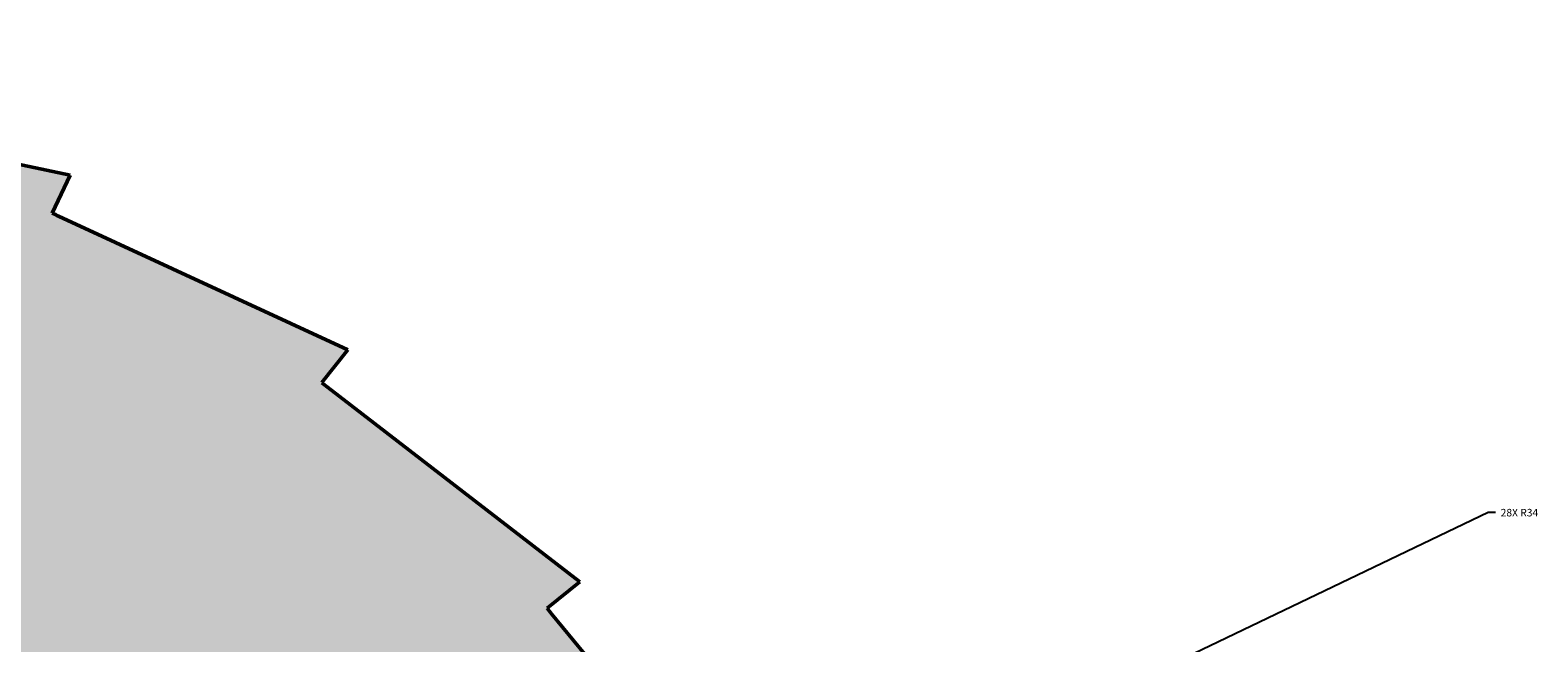
# Model space of a CAD drawing. Units: millimetres. Extents: x 2943.6 to 3032.7, y 1562 to 1639.7.
# Tile 9 of 9: x 2996.7 to 3032.7, y 1621.2 to 1635.8. Entities that reach past the tile are written whole.
import ezdxf

# ---------------------------------------------------------------- set-up
doc = ezdxf.new("R2010")
doc.units = ezdxf.units.MM
doc.layers.add('M-DIMS', color=2, linetype='Continuous', lineweight=18)
doc.layers.add('M-OUTL', color=7, linetype='Continuous', lineweight=50)
doc.layers.add('M-HATC', color=7, linetype='Continuous', lineweight=18, true_color=0xffffff)
doc.styles.get("Standard").update_dxf_attribs({"font": 'arial.ttf'})
doc.dimstyles.get("Standard").update_dxf_attribs({"dimtxt": 0.18, "dimasz": 0.18, "dimexe": 0.18, "dimexo": 0.0625, "dimgap": 0.09, "dimtad": 0, "dimtih": 1, "dimtoh": 1, "dimdec": 4, "dimzin": 0, "dimdsep": 46, "dimtxsty": 'Standard', "dimcen": 0.09, "dimadec": 0, "dimazin": 0, "dimtfac": 1, "dimtdec": 4, "dimtofl": 0, "dimtmove": 0, "dimatfit": 3, "dimfxl": 1, "dimtolj": 1, "dimtzin": 0, "dimarcsym": 0})

# ---------------------------------------------------------------- blocks, each defined once
blk = doc.blocks.new('*D10')
at = {"layer": 'Defpoints', "color": 0, "transparency": 16777216}
for p in [(3013.14, 1615.522), (2982.469, 1600.848)]:
    blk.add_point(p, dxfattribs=at)
at = {"layer": 'M-DIMS', "color": 0, "lineweight": -2, "transparency": 16777216}
for p, q in [((3031.542, 1624.326), (3013.302, 1615.6)), ((3031.722, 1624.326), (3031.542, 1624.326)), ((2982.379, 1600.848), (2982.559, 1600.848)), ((2982.469, 1600.758), (2982.469, 1600.938))]:
    blk.add_line(p, q, dxfattribs=at)
at = {"layer": 'M-DIMS', "color": 0, "transparency": 16777216}
blk.add_solid([(3013.289, 1615.627), (3013.315, 1615.573), (3013.14, 1615.522)], dxfattribs=at)
at = {"layer": 'M-DIMS', "color": 0, "transparency": 16777216, "insert": (3032.292, 1624.326), "char_height": 0.18, "attachment_point": 5}
blk.add_mtext('\\A1;28X R34', dxfattribs=at)

msp = doc.modelspace()

# ---------------------------------------------------------------- hatches: boundary and pattern name
at = {"layer": 'M-HATC'}
h = msp.add_hatch(color=256, dxfattribs=at)
h.set_gradient(color1=(0, 0, 255), color2=(255, 255, 0), tint=1, name='INVCURVED')
h.paths.add_polyline_path([(2949.361, 1608.583, 0.001279), (2949.322, 1608.414), (2948.347, 1608.637), (2948.473, 1600.848), (2947.469, 1600.848), (2949.283, 1593.452, 0.001279), (2949.322, 1593.283), (2948.347, 1593.06), (2951.761, 1586.253, 0.001279), (2951.836, 1586.096), (2950.935, 1585.662), (2955.779, 1579.786, 0.001279), (2955.887, 1579.65), (2955.105, 1579.026), (2961.135, 1574.375, 0.001279), (2961.271, 1574.266), (2960.647, 1573.484), (2967.561, 1570.291, 0.001279), (2967.717, 1570.215), (2967.283, 1569.314), (2974.734, 1567.74, 0.001279), (2974.904, 1567.701), (2974.681, 1566.726), (2982.295, 1566.849, 0.001279), (2982.469, 1566.848), (2982.469, 1565.848), (2989.865, 1567.662, 0.001279), (2990.035, 1567.701), (2990.258, 1566.726), (2997.064, 1570.14, 0.001279), (2997.221, 1570.215), (2997.655, 1569.314), (3003.532, 1574.158, 0.001279), (3003.668, 1574.266), (3004.291, 1573.484), (3008.943, 1579.514, 0.001279), (3009.052, 1579.65), (3009.833, 1579.026), (3013.026, 1585.94, 0.001279), (3013.102, 1586.096), (3014.003, 1585.662), (3015.578, 1593.113, 0.001279), (3015.617, 1593.283), (3016.592, 1593.06), (3016.469, 1600.674, 0.001279), (3016.469, 1600.848), (3017.469, 1600.848), (3015.655, 1608.244, 0.001279), (3015.617, 1608.414), (3016.592, 1608.637), (3013.177, 1615.443, 0.001279), (3013.102, 1615.6), (3014.003, 1616.034), (3009.16, 1621.911, 0.001279), (3009.052, 1622.047), (3009.833, 1622.67), (3003.804, 1627.322, 0.001279), (3003.668, 1627.431), (3004.291, 1628.212), (2997.378, 1631.405, 0.001279), (2997.221, 1631.481), (2997.655, 1632.382), (2990.204, 1633.957, 0.001279), (2990.035, 1633.996), (2990.258, 1634.971), (2982.469, 1634.845), (2982.469, 1635.848), (2975.073, 1634.034, 0.001279), (2974.904, 1633.996), (2974.681, 1634.971), (2967.874, 1631.556, 0.001279), (2967.717, 1631.481), (2967.283, 1632.382), (2961.407, 1627.539, 0.001279), (2961.271, 1627.431), (2960.647, 1628.212), (2955.996, 1622.183, 0.001279), (2955.887, 1622.047), (2955.105, 1622.67), (2951.912, 1615.757, 0.001279), (2951.836, 1615.6), (2950.935, 1616.034)])
h.paths.add_polyline_path([(2969.149, 1610.848, -1), (2961.149, 1610.848, -1)], flags=16)
h.paths.add_polyline_path([(2969.149, 1590.848, -1), (2961.149, 1590.848, -1)], flags=16)
h.paths.add_polyline_path([(2992.469, 1600.848, -1), (2972.469, 1600.848, -1)], flags=16)
h.paths.add_polyline_path([(2978.469, 1620.848, -1), (2986.469, 1620.848, -1)], flags=16)
h.paths.add_polyline_path([(2981.469, 1605.236), (2981.469, 1606.848), (2983.469, 1606.848), (2983.469, 1605.236, -8.887482)], flags=0)
h.paths.add_polyline_path([(2986.469, 1580.848, -1), (2978.469, 1580.848, -1)], flags=16)
h.paths.add_polyline_path([(3003.79, 1610.848, -1), (2995.79, 1610.848, -1)], flags=16)
h.paths.add_polyline_path([(3003.79, 1590.848, -1), (2995.79, 1590.848, -1)], flags=16)

# ---------------------------------------------------------------- linework, layer by layer
at = {"layer": 'M-OUTL'}
for p, q in [((2990.204, 1633.957), (2997.655, 1632.382)), ((2997.221, 1631.481), (2997.655, 1632.382)), ((2997.378, 1631.405), (3004.291, 1628.212)), ((3003.668, 1627.431), (3004.291, 1628.212)), ((3003.804, 1627.322), (3009.833, 1622.67)), ((3009.052, 1622.047), (3009.833, 1622.67)), ((3009.16, 1621.911), (3014.003, 1616.034))]:
    msp.add_line(p, q, dxfattribs=at)
for start, end in [(63.9926, 64.2857), (51.1355, 51.4286), (38.2783, 38.5714)]:
    msp.add_arc((2982.469, 1600.848), 34, start, end, dxfattribs=at)

# ---------------------------------------------------------------- dimensions: what is measured, and where the dimension line sits
at = {"layer": 'M-DIMS'}
dim = msp.add_radius_dim(center=(2982.469, 1600.848), mpoint=(3013.14, 1615.522), text='28X <>', dimstyle='Standard', override={"dimdec": 0, "dimlfac": 1, "dimrnd": 0, "dimzin": 0, "dimdsep": 46, "dimlunit": 2}, dxfattribs=at)
dim.commit()
dim.dimension.update_dxf_attribs({"geometry": '*D10', "text_midpoint": (3032.292, 1624.326), "dimtype": 164})

doc.saveas('drawing.dxf')
